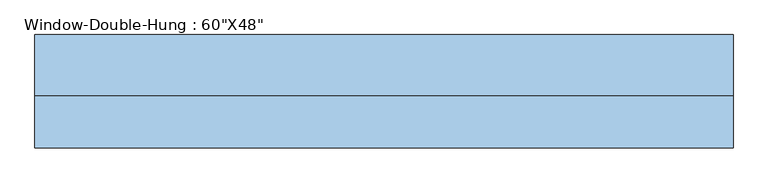
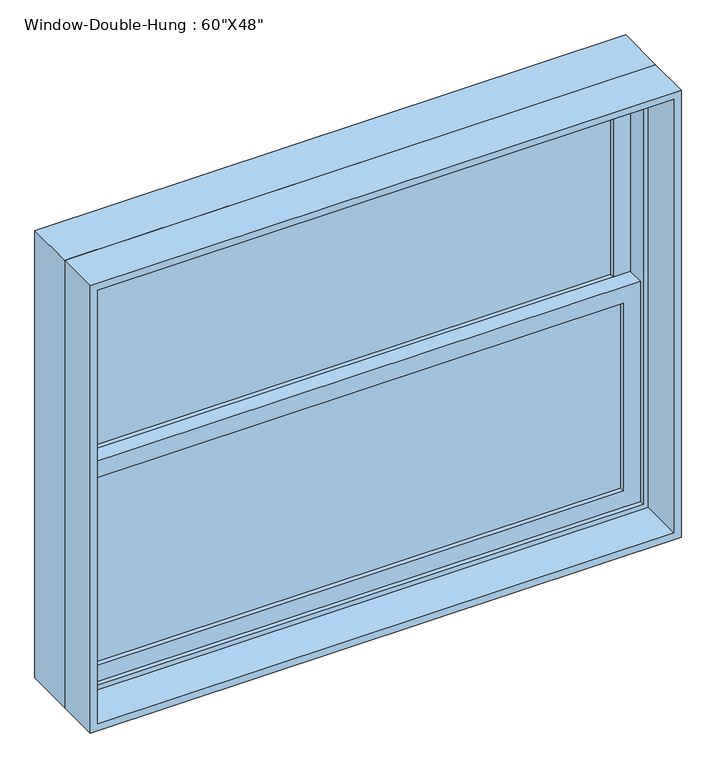
"""IFC4 building model written with IfcOpenShell, lengths in millimetres: window geometry."""

from ifc_helpers import new_model, si_unit, frame, origin, place, context, project, spatial, polyline, outline, extrude, source, transform, mapped, element, save


def window_a144fa31(model_context):
    return source(origin(), model_context, "Body", "SweptSolid", [
        extrude(outline(polyline([(685.8, 44.45), (685.8, 38.1), (-685.8, 38.1), (-685.8, 44.45), (685.8, 44.45)])), frame((0.0, 0.0, 990.6), z_axis=(0.0, 0.0, 1.0), x_axis=(1.0, 0.0, 0.0)), (0.0, 0.0, 1.0), 511.175),
        extrude(outline(polyline([(-685.8, 31.75), (685.8, 31.75), (685.8, 25.4), (-685.8, 25.4), (-685.8, 31.75)])), frame((0.0, 0.0, 990.6), z_axis=(0.0, 0.0, 1.0), x_axis=(1.0, 0.0, 0.0)), (0.0, 0.0, 1.0), 511.175),
        extrude(outline(polyline([(685.8, 88.9), (685.8, 82.55), (-685.8, 82.55), (-685.8, 88.9), (685.8, 88.9)])), frame((0.0, 0.0, 1546.225), z_axis=(0.0, 0.0, 1.0), x_axis=(1.0, 0.0, 0.0)), (0.0, 0.0, 1.0), 511.175),
        extrude(outline(polyline([(-685.8, 76.2), (685.8, 76.2), (685.8, 69.85), (-685.8, 69.85), (-685.8, 76.2)])), frame((0.0, 0.0, 1546.225), z_axis=(0.0, 0.0, 1.0), x_axis=(1.0, 0.0, 0.0)), (0.0, 0.0, 1.0), 511.175),
        extrude(outline(polyline([(1546.225, -730.25), (946.15, -730.25), (946.15, 730.25), (1546.225, 730.25), (1546.225, -730.25)]), holes=[polyline([(1501.775, 685.8), (990.6, 685.8), (990.6, -685.8), (1501.775, -685.8), (1501.775, 685.8)])]), frame((0.0, 12.7, 0.0), z_axis=(0.0, 1.0, 0.0), x_axis=(0.0, 0.0, 1.0)), (0.0, 0.0, 1.0), 44.45),
        extrude(outline(polyline([(2101.85, -730.25), (1501.775, -730.25), (1501.775, 730.25), (2101.85, 730.25), (2101.85, -730.25)]), holes=[polyline([(2057.4, 685.8), (1546.225, 685.8), (1546.225, -685.8), (2057.4, -685.8), (2057.4, 685.8)])]), frame((0.0, 57.15, 0.0), z_axis=(0.0, 1.0, 0.0), x_axis=(0.0, 0.0, 1.0)), (0.0, 0.0, 1.0), 44.45),
        extrude(outline(polyline([(2133.6, -762.0), (914.4, -762.0), (914.4, 762.0), (2133.6, 762.0), (2133.6, -762.0)]), holes=[polyline([(2101.85, 730.25), (946.15, 730.25), (946.15, -730.25), (2101.85, -730.25), (2101.85, 730.25)])]), frame((0.0, 0.0, 0.0), z_axis=(0.0, 1.0, 0.0), x_axis=(0.0, 0.0, 1.0)), (0.0, 0.0, 1.0), 133.35),
        extrude(outline(polyline([(2133.6, 762.0), (2133.6, -762.0), (914.4, -762.0), (914.4, 762.0), (2133.6, 762.0)]), holes=[polyline([(2114.55, 742.95), (933.45, 742.95), (933.45, -742.95), (2114.55, -742.95), (2114.55, 742.95)])]), frame((0.0, -114.3, 0.0), z_axis=(0.0, 1.0, 0.0), x_axis=(0.0, 0.0, 1.0)), (0.0, 0.0, 1.0), 114.3),
    ])


if __name__ == "__main__":
    model = new_model("IFC4")
    model_context = context("Model", 3, world=origin())
    ifc_project = project(units=[si_unit("LENGTHUNIT", "METRE", prefix="MILLI")], contexts=[model_context])
    site = spatial("IfcSite", under=ifc_project)
    building = spatial("IfcBuilding", under=site)
    placement = place(None, origin())
    window_shape = window_a144fa31(model_context)
    element("IfcWindow", 1, ObjectType="Window-Double-Hung : 60\"X48\"", at=placement, inside=building, context=model_context, shape_type="MappedRepresentation", body=[
        mapped(window_shape, transform((0.0, 0.0, 0.0), x_axis=(1.0, 0.0, 0.0), y_axis=(0.0, 1.0, 0.0), z_axis=(0.0, 0.0, 1.0))),
    ])
    save(model, "model.ifc")

# Revit data of these elements
# Type "Window-Double-Hung : 60\"X48\""
#   Type Mark = "18"
#   Fire Rating = "0.5h"
#   Construction Type Id = "DG-DR"
#   Assembly Code = "B2020100"
#   Analytic Construction = "Double glazing - domestic"
#   Wall Thickness [instance default] = 0' - 6"
#   Window Inset [instance default] = 0' - 0"
#   Visual Light Transmittance = 0.81
#   Thermal Resistance (R) = 1.8146 (h·ft²·°F)/BTU
#   Solar Heat Gain Coefficient = 0.76
#   Muntin Width = 4' - 6"
#   Muntin Height = 1' - 8 1/8"
#   Interior Wall Closure [instance default] = 0' - 1 1/2"
#   Rough Width = 5' - 0 1/2"
#   Rough Height = 4' - 0 1/2"
#   Frame Extension [instance default] = 0' - 1 1/4"
#   Exterior Wall Closure [instance default] = 0' - 0 1/2"
#   Extension Jamb [instance default] = 0' - 1 1/2"
#   Heat Transfer Coefficient (U) = 0.5511 BTU/(h·ft²·°F)
#   Height = 4' - 0"
#   Width = 5' - 0"
#   Top Muntin Visibility = yes
#   Indicator Visibility [instance default] = yes
#   Extension Jamb Visibility [instance default] = yes
#   Interior Trim Visibility [instance default] = yes
#   Exterior Trim Visibility [instance default] = yes
#   Define Thermal Properties by = 1
#   Bottom Muntin Visibility = yes
#   Muntin Pattern = Muntin Pattern_2x2 : Muntin Pattern_2x2
#   Interior Trim Material = Wood - Stained
#   Interior Trim = Trim-Window-Interior-Flat : Picture Frame
#   Exterior Trim Material = Clad - White
#   Exterior Trim = Trim-Window-Exterior-Flat : with Sill
#   Glass Panel Material = Glass
#   Exterior Frame Material = Clad - White
#   Interior Frame Material = Wood - Stained
#   Wall Closure = (empty or 0)
# Element 1 (IfcWindow, "Window-Double-Hung : 60\"X48\"")
#   Wall Thickness = 0' - 9"
#   Extension Jamb = 0' - 4 1/2"
#   Materials on its faces: "Wood - Stained", "Glass", "Clad - White"
# Materials
#   "Wood - Stained": class "Wood", colour RGB 224 178 126, transparency 0, Cost = 0
#   "Clad - White": class "Wood", colour RGB 242 242 238, transparency 0, Cost = 0
#   "Glass": class "Glass", colour RGB 0 128 192, transparency 0.75, Description = "Soda Lime Glass", Cost = 0
